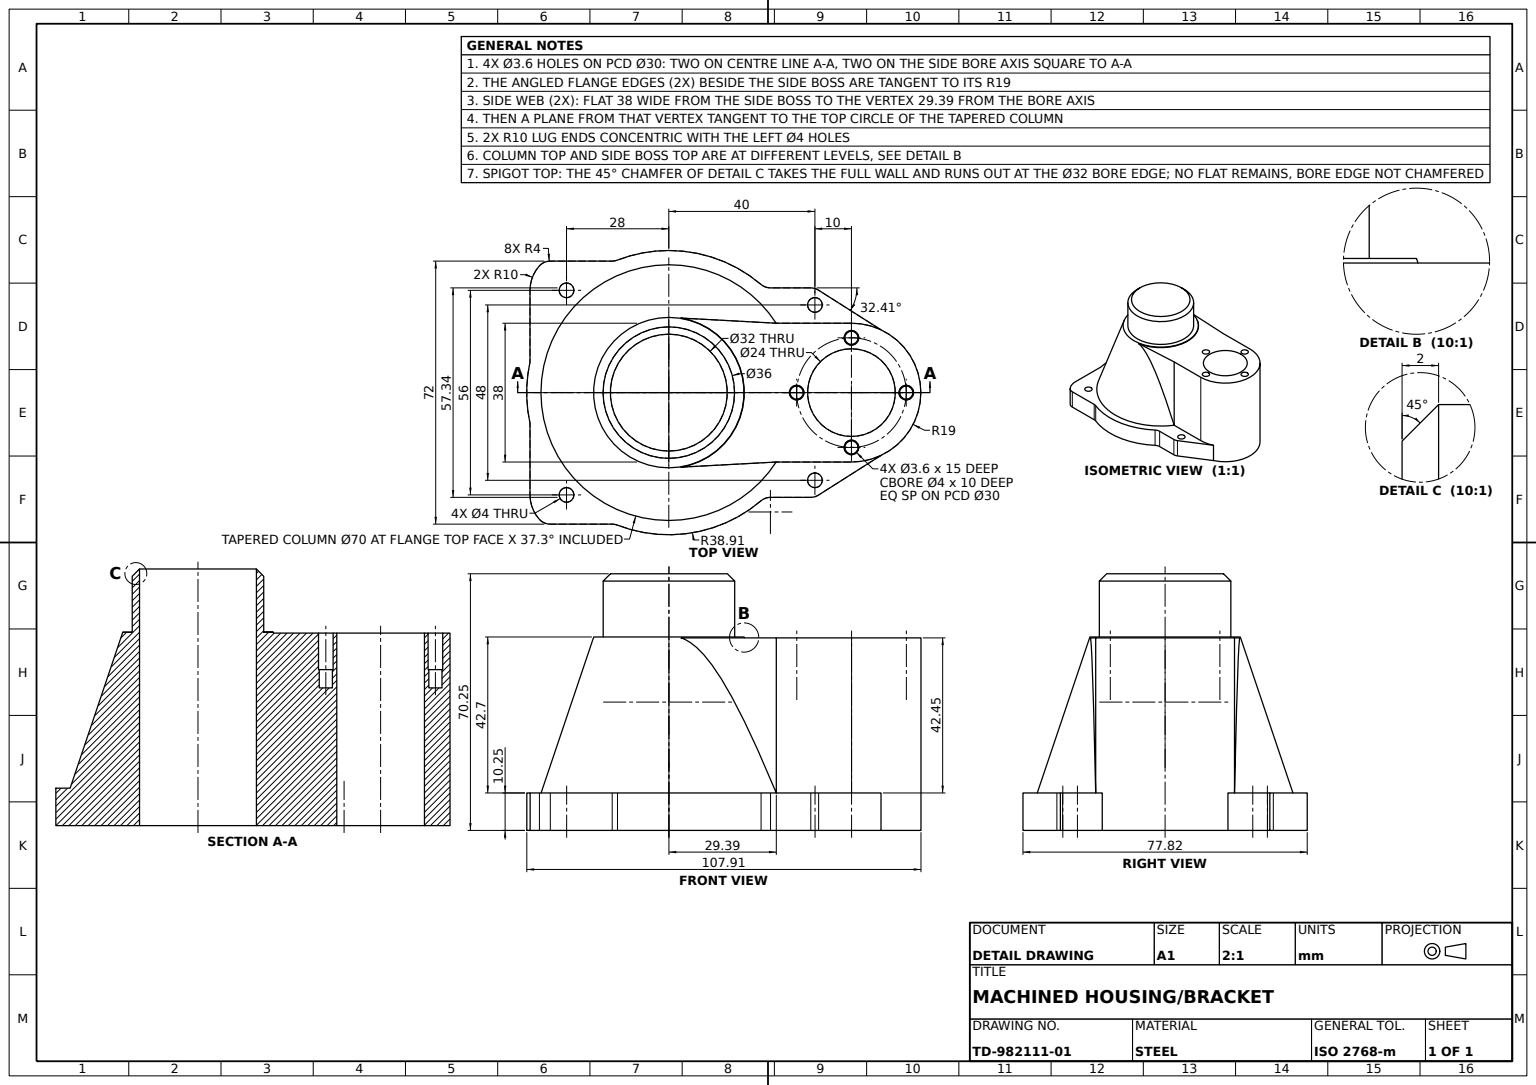
from build123d import *

# Parameters (mm, degrees)
BASE_FLANGE_DEPTH                 = 10.25
TAPERED_COLUMN_SKETCH_R           = 35
TAPERED_COLUMN_DEPTH              = 42.7
TAPERED_COLUMN_TAPER              = 18.65
TOP_BOSS_SKETCH_R                 = 18
TOP_BOSS_DEPTH                    = 15.3
TOP_COLLAR_SKETCH_R               = 18
TOP_COLLAR_45DEG_TAPER_DEPTH      = 2
TOP_COLLAR_45DEG_TAPER_TAPER      = 45
SIDE_BOSS_DEPTH                   = 42.45
SIDE_BOSS_HOLES_SKETCH_R          = 2
SIDE_BOSS_HOLES_4X_DEPTH_10_DEPTH = 10
SECONDARY_HOLES_SKETCH_R          = 1.8
SECONDARY_HOLES_4X_DEPTH_5_DEPTH  = 5
SIDE_BORE_SKETCH_R                = 12
SIDE_BORE_DEPTH                   = 177
MAIN_BORE_SKETCH_R                = 16
MAIN_BORE_DEPTH                   = 177
FLANGE_HOLES_SKETCH_R             = 2
FLANGE_HOLES_4X_DEPTH             = 177


with BuildPart() as part:
    # Base Flange Sketch → Base Flange (new body)
    with BuildSketch(Plane(origin=(0, 0, 0), x_dir=(1, 0, 0), z_dir=(0, 1, 0))):
        with BuildLine():
            Line((58.058170092, 17.206565455), (40.981411355, 28.048001668))
            ThreePointArc((40.981411355, 28.048001668), (39.953813512, 28.512142384), (38.837512739, 28.671065375))
            Line((38.837512739, 28.671065375), (27.817939746, 28.671065375))
            ThreePointArc((27.817939746, 28.671065375), (26.436324443, 28.917248763), (25.224774509, 29.625495798))
            ThreePointArc((25.224774509, 29.625495798), (6.486223775, 38.365194531), (-14.083923128, 36.271233224))
            ThreePointArc((-14.083923128, 36.271233224), (-14.795259826, 36.068393006), (-15.531783042, 36))
            Line((-15.531783042, 36), (-28, 36))
            Line((-28, 36), (-32.472135955, 36))
            ThreePointArc((-32.472135955, 36), (-34.105129117, 35.651483717), (-35.453559925, 34.666666667))
            ThreePointArc((-35.453559925, 34.666666667), (-37.34172359, 31.568220898), (-38, 28))
            Line((-38, 28), (-38, 8.364164649))
            ThreePointArc((-38, 8.364164649), (-38.909629274, 0), (-38, -8.364164649))
            Line((-38, -8.364164649), (-38, -28))
            ThreePointArc((-38, -28), (-37.34172359, -31.568220898), (-35.453559925, -34.666666667))
            ThreePointArc((-35.453559925, -34.666666667), (-34.105129117, -35.651483717), (-32.472135955, -36))
            Line((-32.472135955, -36), (-28, -36))
            Line((-28, -36), (-15.531783042, -36))
            ThreePointArc((-15.531783042, -36), (-14.795259826, -36.068393006), (-14.083923128, -36.271233224))
            ThreePointArc((-14.083923128, -36.271233224), (6.486223775, -38.365194531), (25.224774509, -29.625495798))
            ThreePointArc((25.224774509, -29.625495798), (26.436324443, -28.917248763), (27.817939746, -28.671065375))
            Line((27.817939746, -28.671065375), (38.837512739, -28.671065375))
            ThreePointArc((38.837512739, -28.671065375), (39.953813512, -28.512142384), (40.981411355, -28.048001668))
            Line((40.981411355, -28.048001668), (58.058170092, -17.206565455))
            ThreePointArc((58.058170092, -17.206565455), (69, 0), (58.058170092, 17.206565455))
        make_face()
    extrude(amount=BASE_FLANGE_DEPTH)

    # Tapered Column Sketch → Tapered Column (add)
    with BuildSketch(Plane(origin=(0, 10.25, 0), x_dir=(1, 0, 0), z_dir=(0, 1, 0))):
        Circle(TAPERED_COLUMN_SKETCH_R)
    extrude(amount=TAPERED_COLUMN_DEPTH, taper=TAPERED_COLUMN_TAPER)

    # Top Boss Sketch → Top Boss (add)
    with BuildSketch(Plane(origin=(0, 52.95, 0), x_dir=(1, 0, 0), z_dir=(0, 1, 0))):
        with Locations(Location((0, 0, 0), (0, 0, 270))):
            Circle(TOP_BOSS_SKETCH_R)
    extrude(amount=TOP_BOSS_DEPTH)

    # Top Collar Sketch → Top Collar 45deg Taper (add)
    with BuildSketch(Plane(origin=(0, 68.25, 0), x_dir=(1, 0, 0), z_dir=(0, 1, 0))):
        with Locations(Location((0, 0, 0), (0, 0, 270))):
            Circle(TOP_COLLAR_SKETCH_R)
    extrude(amount=TOP_COLLAR_45DEG_TAPER_DEPTH, taper=TOP_COLLAR_45DEG_TAPER_TAPER)

    # Side Boss Sketch → Side Boss (add)
    with BuildSketch(Plane(origin=(0, 10.25, 0), x_dir=(1, 0, 0), z_dir=(0, 1, 0))):
        with BuildLine():
            ThreePointArc((50, -19), (69, 0), (50, 19))
            Line((50, 19), (29.393876913, 19))
            Line((29.393876913, 19), (2.218603036, 20.468479678))
            ThreePointArc((2.218603036, 20.468479678), (20.588367098, 0), (2.218603036, -20.468479678))
            Line((2.218603036, -20.468479678), (29.393876913, -19))
            Line((29.393876913, -19), (50, -19))
        make_face()
    extrude(amount=SIDE_BOSS_DEPTH)

    # Side Boss Holes Sketch → Side Boss Holes 4x Depth 10 (cut)
    with BuildSketch(Plane(origin=(0, 52.7, 0), x_dir=(1, 0, 0), z_dir=(0, 1, 0))):
        with Locations(Location((35, 0, 0), (0, 0, 270))):
            Circle(SIDE_BOSS_HOLES_SKETCH_R)
        with Locations(Location((50, 15, 0), (0, 0, 270))):
            Circle(SIDE_BOSS_HOLES_SKETCH_R)
        with Locations(Location((65, 0, 0), (0, 0, 270))):
            Circle(SIDE_BOSS_HOLES_SKETCH_R)
        with Locations(Location((50, -15, 0), (0, 0, 270))):
            Circle(SIDE_BOSS_HOLES_SKETCH_R)
    extrude(amount=-SIDE_BOSS_HOLES_4X_DEPTH_10_DEPTH, mode=Mode.SUBTRACT)

    # Secondary Holes Sketch → Secondary Holes 4x Depth 5 (cut)
    with BuildSketch(Plane(origin=(0, 42.7, 0), x_dir=(1, 0, 0), z_dir=(0, 1, 0))):
        with Locations(Location((35, 0, 0), (0, 0, 270))):
            Circle(SECONDARY_HOLES_SKETCH_R)
        with Locations(Location((65, 0, 0), (0, 0, 270))):
            Circle(SECONDARY_HOLES_SKETCH_R)
        with Locations(Location((50, -15, 0), (0, 0, 270))):
            Circle(SECONDARY_HOLES_SKETCH_R)
        with Locations(Location((50, 15, 0), (0, 0, 270))):
            Circle(SECONDARY_HOLES_SKETCH_R)
    extrude(amount=-SECONDARY_HOLES_4X_DEPTH_5_DEPTH, mode=Mode.SUBTRACT)

    # Side Bore Sketch → Side Bore (cut)
    with BuildSketch(Plane(origin=(0, 52.7, 0), x_dir=(1, 0, 0), z_dir=(0, 1, 0))):
        with Locations(Location((50, 0, 0), (0, 0, 270))):
            Circle(SIDE_BORE_SKETCH_R)
    extrude(amount=-SIDE_BORE_DEPTH, mode=Mode.SUBTRACT)

    # Main Bore Sketch → Main Bore (cut)
    with BuildSketch(Plane(origin=(0, 70.25, 0), x_dir=(1, 0, 0), z_dir=(0, 1, 0))):
        with Locations(Location((0, 0, 0), (0, 0, 270))):
            Circle(MAIN_BORE_SKETCH_R)
    extrude(amount=-MAIN_BORE_DEPTH, mode=Mode.SUBTRACT)

    # Flange Holes Sketch → Flange Holes 4x (cut)
    with BuildSketch(Plane(origin=(0, 10.25, 0), x_dir=(1, 0, 0), z_dir=(0, 1, 0))):
        with Locations(Location((40, -24, 0), (0, 0, 270))):
            Circle(FLANGE_HOLES_SKETCH_R)
        with Locations(Location((40, 24, 0), (0, 0, 270))):
            Circle(FLANGE_HOLES_SKETCH_R)
        with Locations(Location((-28, 28, 0), (0, 0, 270))):
            Circle(FLANGE_HOLES_SKETCH_R)
        with Locations(Location((-28, -28, 0), (0, 0, 270))):
            Circle(FLANGE_HOLES_SKETCH_R)
    extrude(amount=-FLANGE_HOLES_4X_DEPTH, mode=Mode.SUBTRACT)


solid = part.part
